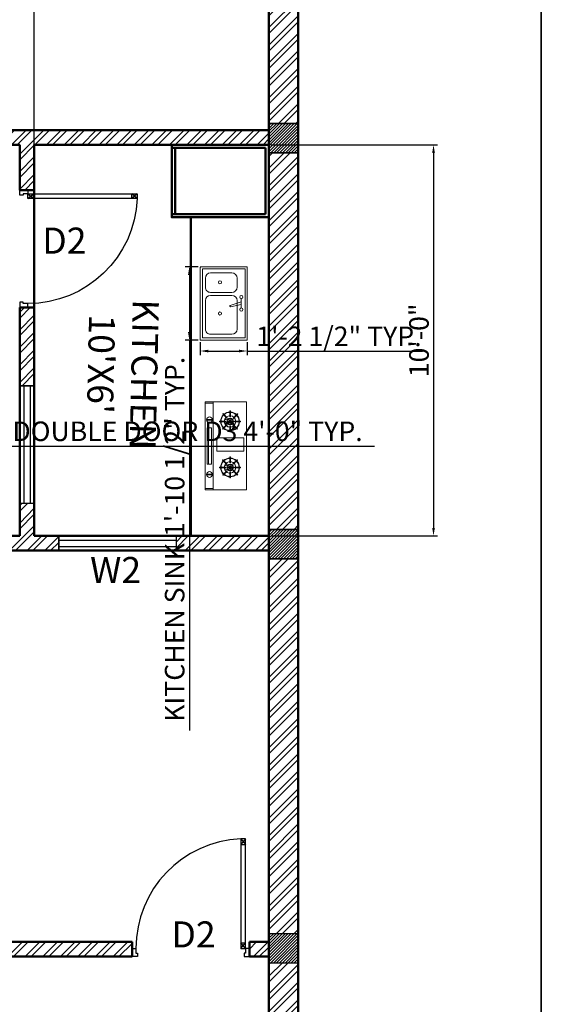
# Model space of a CAD drawing. Units: millimetres. Extents: x 20768 to 23556, y 50760 to 52704.
# Tile 25 of 36: x 21474 to 21634, y 52066 to 52368. Entities that reach past the tile are written whole.
import ezdxf

# ---------------------------------------------------------------- set-up
doc = ezdxf.new("R2010")
doc.units = ezdxf.units.MM
for name, color, linetype, lineweight in [('A-ANNO-TTLB', 7, 'Continuous', 35), ('A-AREA-IDEN', 40, 'Continuous', 18), ('A-DOOR', 3, 'Continuous', 25), ('A-FURN', 8, 'Continuous', 18), ('A-GLAZ', 4, 'Continuous', 25), ('A-WALL', 7, 'Continuous', 50), ('A-WALL-PATT', 8, 'Continuous', 13), ('S-ANNO-DIMS', 2, 'Continuous', 18), ('S-COLS', 20, 'Continuous', 35)]:
    doc.layers.add(name, color=color, linetype=linetype, lineweight=lineweight)
doc.styles.get("Standard").update_dxf_attribs({"font": 'arial.ttf'})
doc.dimstyles.new('ISO-25', dxfattribs={"dimtxt": 6, "dimasz": 2.5, "dimexe": 1.25, "dimexo": 0.625, "dimtad": 1, "dimdec": 0, "dimlunit": 3, "dimtxsty": 'Standard', "dimcen": 2.5, "dimadec": 0, "dimazin": 0, "dimtfac": 1, "dimtdec": 0, "dimtmove": 0, "dimatfit": 3, "dimfxl": 1, "dimarcsym": 0})
pattern_1 = [(45, (-37.4434, 0), (-2.69407684, 2.69407684), []), (45, (-35.6473, 0), (-2.69407684, 2.69407684), [])]
pattern_2 = [(45, (345.4904, 0), (-0.449012806, 0.449012806), [])]

# ---------------------------------------------------------------- blocks, each defined once
blk = doc.blocks.new('Puerta 01')
for p, q in [((-0.7745, -0.0264), (-0.7368, -0.0584)), ((-0.7745, -0.0584), (-0.7368, -0.0264)), ((-0.7368, -0.0584), (-0.7368, -0.0264)), ((-0.028, -0.0584), (-0.0657, -0.0264)), ((-0.028, -0.0264), (-0.0657, -0.0584)), ((-0.0657, -0.0584), (-0.0657, -0.0264))]:
    blk.add_line(p, q)
for points in [[(-0.028, 0), (-0.028, -0.0264), (0.004, -0.0264), (0.004, -0.036), (0.028, -0.036), (0.028, 0)], [(-0.028, -0.0264), (-0.7745, -0.0264), (-0.7745, -0.0584), (-0.028, -0.0584)], [(0.004, -0.7736), (0.004, -0.764), (0.028, -0.764), (0.028, -0.8), (-0.028, -0.8), (-0.028, -0.7736)]]:
    blk.add_lwpolyline(points, close=True)
blk.add_arc((-0.028, -0.0264), 0.7472, 182.45453, 270)
blk = doc.blocks.new('A$C46C9437A')
for p, q in [((0, 416.4), (0, 0.8)), ((884.8, 416.4), (0, 416.4)), ((884.8, 0.8), (884.8, 416.4)), ((163, 281.2), (120.3, 323.9)), ((166.8, 285), (124.1, 327.7)), ((194.5, 296.3), (194.5, 356.7)), ((199.9, 296.2), (199.9, 356.6)), ((228.4, 283.6), (271.1, 326.3)), ((232.1, 279.7), (274.9, 322.4)), ((495.4, 390.2), (361.5, 390.2)), ((361.5, 390.2), (361.5, 118)), ((495.4, 118), (495.4, 390.2)), ((624.8, 279.7), (582.1, 322.4)), ((628.5, 283.6), (585.8, 326.3)), ((657, 296.2), (657, 356.6)), ((662.4, 296.3), (662.4, 356.7)), ((690.1, 285), (732.8, 327.7)), ((693.9, 281.2), (736.6, 323.9)), ((151.4, 249.7), (91, 249.7)), ((151.6, 255.1), (91.1, 255.1)), ((160.6, 223.4), (117.7, 180.6)), ((164.1, 219.3), (121.4, 176.6)), ((171.6, 252.1), (165.7, 252.1)), ((165.7, 252.1), (165.7, 251.1)), ((165.7, 251.1), (171.6, 251.1)), ((171.6, 251.1), (171.6, 252.1)), ((181.4, 195.8), (172.2, 230.6)), ((194.5, 205.4), (194.5, 145)), ((197.3, 281.9), (196.3, 281.9)), ((196.3, 281.9), (196.3, 276.4)), ((196.3, 276.4), (197.3, 276.4)), ((197.3, 226.1), (196.3, 226.1)), ((196.3, 226.1), (196.3, 220.6)), ((196.3, 220.6), (197.3, 220.6)), ((197.3, 276.4), (197.3, 281.9)), ((197.3, 220.6), (197.3, 226.1)), ((199.9, 205.4), (199.9, 145)), ((212, 195.1), (222.8, 232)), ((227.3, 252.1), (221.4, 252.1)), ((221.4, 252.1), (221.4, 251.1)), ((221.4, 251.1), (227.3, 251.1)), ((227.2, 216.9), (269.9, 174.2)), ((227.3, 251.1), (227.3, 252.1)), ((231, 220.8), (273.7, 178.1)), ((242.2, 255.1), (302.6, 255.1)), ((242.4, 249.7), (302.7, 249.7)), ((614.6, 249.7), (554.2, 249.7)), ((614.7, 255.1), (554.3, 255.1)), ((625.9, 220.8), (583.2, 178.1)), ((629.7, 216.9), (587, 174.2)), ((629.6, 251.1), (629.6, 252.1)), ((629.6, 252.1), (635.6, 252.1)), ((635.6, 251.1), (629.6, 251.1)), ((644.9, 195.1), (634.1, 232)), ((635.6, 252.1), (635.6, 251.1)), ((657, 205.4), (657, 145)), ((659.6, 276.4), (659.6, 281.9)), ((659.6, 281.9), (660.7, 281.9)), ((660.7, 276.4), (659.6, 276.4)), ((659.6, 220.6), (659.6, 226.1)), ((659.6, 226.1), (660.7, 226.1)), ((660.7, 220.6), (659.6, 220.6)), ((660.7, 281.9), (660.7, 276.4)), ((660.7, 226.1), (660.7, 220.6)), ((662.4, 205.4), (662.4, 145)), ((675.5, 195.8), (684.7, 230.6)), ((685.3, 251.1), (685.3, 252.1)), ((685.3, 252.1), (691.3, 252.1)), ((691.3, 251.1), (685.3, 251.1)), ((691.3, 252.1), (691.3, 251.1)), ((692.8, 219.3), (735.5, 176.6)), ((696.3, 223.4), (739.2, 180.6)), ((705.3, 255.1), (765.8, 255.1)), ((705.5, 249.7), (765.9, 249.7)), ((361.5, 118), (495.4, 118)), ((0, 82.1), (884.8, 82.1)), ((0, 0.8), (884.8, 0.8)), ((11.9, 0), (11.9, 81.7)), ((184.5, 70.7), (176.8, 70.7)), ((176.8, 70.7), (176.8, 15.6)), ((176.8, 15.6), (184.5, 15.6)), ((184.5, 15.6), (184.5, 70.7)), ((628.6, 65.2), (261.1, 65.2)), ((261.1, 65.2), (261.1, 20.8)), ((628.6, 32.6), (261.1, 32.6)), ((261.1, 20.8), (628.6, 20.8)), ((628.6, 20.8), (628.6, 65.2)), ((735.8, 70.7), (728.1, 70.7)), ((728.1, 70.7), (728.1, 15.6)), ((728.1, 15.6), (735.8, 15.6)), ((735.8, 15.6), (735.8, 70.7)), ((872.3, 0), (872.3, 81.7))]:
    blk.add_line(p, q)
for centre, radius in [((196.7, 251.4), 32.5), ((196.7, 251.4), 30.7), ((173.8, 251.8), 2.11), ((180.2, 236.2), 2.11), ((180.6, 267.5), 2.11), ((196.2, 251.6), 14.5), ((196.2, 251.6), 12.7), ((196, 251.9), 4.75), ((196.7, 274.5), 2.11), ((196.7, 228.2), 2.11), ((211.9, 235.8), 2.11), ((212.3, 267), 2.11), ((218.6, 251.8), 2.11), ((660.3, 251.4), 32.5), ((660.3, 251.4), 30.7), ((638.3, 251.8), 2.11), ((644.6, 267), 2.11), ((645, 235.8), 2.11), ((660.7, 251.6), 14.5), ((660.7, 251.6), 12.7), ((660.9, 251.9), 4.75), ((660.3, 274.5), 2.11), ((660.3, 228.2), 2.11), ((676.3, 267.5), 2.11), ((676.7, 236.2), 2.11), ((683.1, 251.8), 2.11), ((180.1, 43.9), 29), ((731.4, 43.9), 29)]:
    blk.add_circle(centre, radius)
for centre, radius, start, end in [((196.9, 250.8), 94.6, 136.5182, 177.42683), ((196.9, 250.8), 91, 136.57828, 177.32495), ((196.9, 250.8), 105.8, 133.43323, 136.35675), ((196.9, 250.8), 94.6, 91.4483, 133.24678), ((196.9, 250.8), 91, 91.50561, 133.17739), ((196.9, 250.8), 57.2, 92.39717, 175.73928), ((196.5, 239.1), 117.6, 88.37076, 91.29429), ((196.9, 250.8), 94.6, 45.52997, 88.17687), ((196.9, 250.8), 91, 45.55094, 88.10471), ((196.9, 250.8), 57.2, 45.87705, 86.98209), ((196.9, 250.8), 91, 2.67505, 42.14937), ((196.9, 250.8), 94.6, 2.57317, 42.25795), ((196.9, 250.8), 105.8, 42.54967, 45.47362), ((660, 250.8), 94.6, 137.74205, 177.42683), ((660, 250.8), 91, 137.85063, 177.32495), ((660, 250.8), 105.8, 134.52638, 137.45033), ((660, 250.8), 94.6, 91.82313, 134.47003), ((660, 250.8), 91, 91.89529, 134.44906), ((660, 250.8), 57.2, 93.01791, 134.12295), ((660.4, 239.1), 117.6, 88.70571, 91.62924), ((660, 250.8), 94.6, 46.75322, 88.5517), ((660, 250.8), 91, 46.82261, 88.49439), ((660, 250.8), 57.2, 4.26072, 87.60283), ((660, 250.8), 91, 2.67505, 43.42172), ((660, 250.8), 94.6, 2.57317, 43.4818), ((660, 250.8), 105.8, 43.64325, 46.56677), ((208.6, 250.4), 117.6, 177.70057, 180.33206), ((196.9, 250.8), 94.6, 180.69868, 221.19627), ((196.9, 250.8), 91, 180.72632, 221.04554), ((196.9, 250.8), 57.2, 181.15626, 218.6973), ((196.9, 250.8), 45.5, 174.64455, 181.45263), ((196.9, 250.8), 57.2, 224.12295, 267.60283), ((196.9, 250.8), 45.5, 217.07285, 223.89817), ((196.9, 250.8), 45.5, 131.35328, 138.15746), ((196.9, 250.8), 45.5, 86.2077, 93.01198), ((196.9, 250.8), 45.5, 266.98802, 273.7923), ((196.9, 250.8), 57.2, 273.01791, 312.48709), ((196.9, 250.8), 45.5, 311.84254, 318.64672), ((196.9, 250.8), 45.5, 39.2922, 46.10183), ((196.9, 250.8), 57.2, 317.90212, 358.84374), ((196.9, 250.8), 57.2, 4.26072, 40.45928), ((196.9, 250.8), 45.5, 358.54737, 5.35545), ((196.9, 250.8), 91, 316.82261, 359.27368), ((196.9, 250.8), 94.6, 316.75322, 359.30132), ((196.9, 250.8), 105.8, 359.37561, 2.29943), ((660, 250.8), 105.8, 177.70057, 180.62439), ((660, 250.8), 94.6, 180.69868, 223.24678), ((660, 250.8), 91, 180.72632, 223.17739), ((660, 250.8), 57.2, 181.15626, 222.09788), ((660, 250.8), 57.2, 139.54072, 175.73928), ((660, 250.8), 45.5, 174.64455, 181.45263), ((660, 250.8), 57.2, 227.51291, 266.98209), ((660, 250.8), 45.5, 133.89817, 140.7078), ((660, 250.8), 45.5, 221.35328, 228.15746), ((660, 250.8), 45.5, 86.98802, 93.7923), ((660, 250.8), 45.5, 266.2077, 273.01198), ((660, 250.8), 57.2, 272.39717, 315.87705), ((660, 250.8), 45.5, 41.84254, 48.64672), ((660, 250.8), 45.5, 316.10183, 322.92715), ((660, 250.8), 57.2, 321.3027, 358.84374), ((660, 250.8), 45.5, 358.54737, 5.35545), ((660, 250.8), 91, 318.95446, 359.27368), ((660, 250.8), 94.6, 318.80373, 359.30132), ((648.3, 250.4), 117.6, 359.66794, 2.29943), ((196.9, 250.8), 105.8, 221.60119, 224.52638), ((196.9, 250.8), 94.6, 224.47003, 268.5517), ((196.9, 250.8), 91, 224.44906, 268.49439), ((196.9, 250.8), 105.8, 268.70571, 271.62924), ((196.9, 250.8), 91, 271.89529, 313.42172), ((196.9, 250.8), 94.6, 271.82313, 313.4818), ((196.9, 250.8), 105.8, 313.64325, 316.56677), ((660, 250.8), 105.8, 223.43323, 226.35675), ((660, 250.8), 94.6, 226.5182, 268.17687), ((660, 250.8), 91, 226.57828, 268.10471), ((660, 250.8), 105.8, 268.37076, 271.29429), ((660, 250.8), 91, 271.50561, 315.55094), ((660, 250.8), 94.6, 271.4483, 315.52997), ((660, 250.8), 105.8, 315.47362, 318.39881)]:
    blk.add_arc(centre, radius, start, end)
blk = doc.blocks.new('A$C42714C99')
for p, q in [((0, 445), (0, 5)), ((695, 450), (5, 450)), ((20, 430), (20, 20)), ((680, 430), (20, 430)), ((303.8, 392.6), (393.1, 392.6)), ((335.3, 392.6), (369.3, 287.1)), ((360, 392.6), (382, 288.3)), ((680, 20), (680, 430)), ((700, 5), (700, 445)), ((57.3, 98.6), (57.3, 302.2)), ((107.3, 352.2), (194.5, 352.2)), ((244.5, 302.2), (244.5, 98.6)), ((273.1, 98.6), (273.1, 302.2)), ((323.1, 352.2), (594.9, 352.2)), ((644.9, 302.2), (644.9, 98.6)), ((5, 0), (695, 0)), ((20, 20), (680, 20)), ((194.5, 48.6), (107.3, 48.6)), ((594.9, 48.6), (323.1, 48.6))]:
    blk.add_line(p, q)
for centre in [(288.7, 392.6), (408.3, 392.6), (147.5, 188.3), (446.5, 188.3)]:
    blk.add_circle(centre, 15.1)
for centre, radius, start, end in [((5, 445), 5, 90, 180), ((695, 445), 5, 0, 90), ((107.3, 302.2), 50, 90, 180), ((194.5, 302.2), 50, 0, 90), ((323.1, 302.2), 50, 90, 180), ((375.4, 290.3), 6.89, 207.59576, 343.05259), ((594.9, 302.2), 50, 0, 90), ((107.3, 98.6), 50, 180, 270), ((194.5, 98.6), 50, 270, 0), ((323.1, 98.6), 50, 180, 270), ((594.9, 98.6), 50, 270, 0), ((5, 5), 5, 180, 270), ((1, 1), 1, 180, 270), ((695, 5), 5, 270, 0), ((699, 1), 1, 270, 0)]:
    blk.add_arc(centre, radius, start, end)
blk = doc.blocks.new('A$C00DA51E9')
blk.add_blockref('A$C42714C99', (0, 0))
blk = doc.blocks.new('COL-PLAN')
blk.add_line((0, 9), (9, 9))
blk.add_lwpolyline([(9, 9), (0, 9), (0, 0), (9, 0)], close=True)
blk = doc.blocks.new('WIN-PLAN-A')
blk.add_line((36, 4.5), (36, 0))
blk.add_lwpolyline([(36, 4.5), (0, 4.5), (0, 0), (36, 0)], close=True)
blk = doc.blocks.new('*D185')
at = {"layer": 'Defpoints', "color": 0, "transparency": 16777216}
for p in [(21465.84, 52236.99), (21417.84, 52229.79), (21465.84, 52229.79)]:
    blk.add_point(p, dxfattribs=at)
at = {"layer": 'S-ANNO-DIMS', "color": 0, "lineweight": -2, "transparency": 16777216}
for p, q in [((21417.84, 52230.42), (21417.84, 52238.24)), ((21465.84, 52230.42), (21465.84, 52238.24)), ((21420.34, 52236.99), (21463.34, 52236.99)), ((21465.84, 52236.99), (21583.18, 52236.99))]:
    blk.add_line(p, q, dxfattribs=at)
at = {"layer": 'S-ANNO-DIMS', "color": 0, "transparency": 16777216}
for points in [[(21420.34, 52237.41), (21420.34, 52236.58), (21417.84, 52236.99)], [(21463.34, 52237.41), (21463.34, 52236.58), (21465.84, 52236.99)]]:
    blk.add_solid(points, dxfattribs=at)
at = {"layer": 'S-ANNO-DIMS', "color": 0, "transparency": 16777216, "insert": (21525.76, 52240.73), "char_height": 6, "attachment_point": 5}
blk.add_mtext('DOUBLE DOOR D3 4\'-0" TYP.', dxfattribs=at)
blk = doc.blocks.new('*D195')
at = {"layer": 'Defpoints', "color": 0, "transparency": 16777216}
for p in [(21529.68, 52291.94), (21526.32, 52269.49), (21529.68, 52269.49)]:
    blk.add_point(p, dxfattribs=at)
at = {"layer": 'S-ANNO-DIMS', "color": 0, "lineweight": -2, "transparency": 16777216}
for p, q in [((21529.06, 52291.94), (21525.07, 52291.94)), ((21526.32, 52289.44), (21526.32, 52271.99)), ((21529.06, 52269.49), (21525.07, 52269.49)), ((21526.32, 52269.49), (21526.32, 52149.78))]:
    blk.add_line(p, q, dxfattribs=at)
at = {"layer": 'S-ANNO-DIMS', "color": 0, "transparency": 16777216}
for points in [[(21525.9, 52289.44), (21526.73, 52289.44), (21526.32, 52291.94)], [(21525.9, 52271.99), (21526.73, 52271.99), (21526.32, 52269.49)]]:
    blk.add_solid(points, dxfattribs=at)
at = {"layer": 'S-ANNO-DIMS', "color": 0, "transparency": 16777216, "insert": (21522.59, 52208.39), "char_height": 6, "attachment_point": 5, "rotation": 90}
blk.add_mtext('KITCHEN SINK 1\'-10 1/2" TYP.', dxfattribs=at)
blk = doc.blocks.new('*D196')
at = {"layer": 'Defpoints', "color": 0, "transparency": 16777216}
for p in [(21529.68, 52269.49), (21544.11, 52269.49), (21544.11, 52266.13)]:
    blk.add_point(p, dxfattribs=at)
at = {"layer": 'S-ANNO-DIMS', "color": 0, "lineweight": -2, "transparency": 16777216}
for p, q in [((21529.68, 52268.87), (21529.68, 52264.88)), ((21544.11, 52268.87), (21544.11, 52264.88)), ((21532.18, 52266.13), (21541.61, 52266.13)), ((21544.11, 52266.13), (21597.85, 52266.13))]:
    blk.add_line(p, q, dxfattribs=at)
at = {"layer": 'S-ANNO-DIMS', "color": 0, "transparency": 16777216}
for points in [[(21532.18, 52266.54), (21532.18, 52265.71), (21529.68, 52266.13)], [(21541.61, 52266.54), (21541.61, 52265.71), (21544.11, 52266.13)]]:
    blk.add_solid(points, dxfattribs=at)
at = {"layer": 'S-ANNO-DIMS', "color": 0, "transparency": 16777216, "insert": (21572.23, 52269.85), "char_height": 6, "attachment_point": 5}
blk.add_mtext('1\'-2 1/2" TYP.', dxfattribs=at)
blk = doc.blocks.new('*D214')
at = {"layer": 'Defpoints', "color": 0, "transparency": 16777216}
for p in [(21550.74, 52329.4), (21550.74, 52209.4), (21601.27, 52209.4)]:
    blk.add_point(p, dxfattribs=at)
at = {"layer": 'S-ANNO-DIMS', "color": 0, "lineweight": -2, "transparency": 16777216}
for p, q in [((21551.37, 52329.4), (21602.52, 52329.4)), ((21601.27, 52326.9), (21601.27, 52211.9)), ((21551.37, 52209.4), (21602.52, 52209.4))]:
    blk.add_line(p, q, dxfattribs=at)
at = {"layer": 'S-ANNO-DIMS', "color": 0, "transparency": 16777216}
for points in [[(21600.86, 52326.9), (21601.69, 52326.9), (21601.27, 52329.4)], [(21600.86, 52211.9), (21601.69, 52211.9), (21601.27, 52209.4)]]:
    blk.add_solid(points, dxfattribs=at)
at = {"layer": 'S-ANNO-DIMS', "color": 0, "transparency": 16777216, "insert": (21597.58, 52269.4), "char_height": 6, "attachment_point": 5, "rotation": 90}
blk.add_mtext('10\'-0"', dxfattribs=at)
blk = doc.blocks.new('*D216')
at = {"layer": 'Defpoints', "color": 0, "transparency": 16777216}
for p in [(21550.74, 52564.4), (21478.74, 52209.4), (21550.74, 52209.4)]:
    blk.add_point(p, dxfattribs=at)
at = {"layer": 'S-ANNO-DIMS', "color": 0, "lineweight": -2, "transparency": 16777216}
for p, q in [((21478.74, 52210.02), (21478.74, 52565.65)), ((21481.24, 52564.4), (21548.24, 52564.4)), ((21550.74, 52210.02), (21550.74, 52565.65))]:
    blk.add_line(p, q, dxfattribs=at)
at = {"layer": 'S-ANNO-DIMS', "color": 0, "transparency": 16777216}
for points in [[(21481.24, 52564.81), (21481.24, 52563.98), (21478.74, 52564.4)], [(21548.24, 52564.81), (21548.24, 52563.98), (21550.74, 52564.4)]]:
    blk.add_solid(points, dxfattribs=at)
at = {"layer": 'S-ANNO-DIMS', "color": 0, "transparency": 16777216, "insert": (21514.74, 52568.09), "char_height": 6, "attachment_point": 5}
blk.add_mtext('6\'-0"', dxfattribs=at)

msp = doc.modelspace()

# ---------------------------------------------------------------- hatches: boundary and pattern name
at = {"layer": 'A-WALL-PATT'}
h = msp.add_hatch(dxfattribs=at)
h.set_pattern_fill('ANSI32', color=256, scale=0.4)
h.set_pattern_definition(pattern_1)
h.paths.add_polyline_path([(21559.74, 52513.9), (21550.74, 52513.9), (21550.74, 52335.9), (21559.74, 52335.9)])
h = msp.add_hatch(dxfattribs=at)
h.set_pattern_fill('ANSI31', color=256, scale=0.2)
h.set_pattern_definition(pattern_2)
h.paths.add_polyline_path([(21559.74, 52335.9), (21550.74, 52335.9), (21550.74, 52326.9), (21559.74, 52326.9)])
h = msp.add_hatch(dxfattribs=at)
h.set_pattern_fill('ANSI32', color=256, scale=0.4)
h.set_pattern_definition(pattern_1)
h.paths.add_polyline_path([(21550.74, 52333.9), (21444.64, 52333.9), (21444.64, 52329.4), (21474.24, 52329.4), (21474.24, 52315.5), (21476.76, 52315.5), (21478.74, 52315.5), (21478.74, 52329.4), (21550.74, 52329.4)])
h = msp.add_hatch(dxfattribs=at)
h.set_pattern_fill('ANSI32', color=256, scale=0.4)
h.set_pattern_definition(pattern_1)
h.paths.add_polyline_path([(21559.74, 52326.9), (21550.74, 52326.9), (21550.74, 52307.13), (21550.74, 52211.4), (21559.74, 52211.4)])
h = msp.add_hatch(dxfattribs=at)
h.set_pattern_fill('ANSI32', color=256, scale=0.4)
h.set_pattern_definition(pattern_1)
h.paths.add_polyline_path([(21478.74, 52279.5), (21474.24, 52279.5), (21474.24, 52255.5), (21478.74, 52255.5)])
h = msp.add_hatch(dxfattribs=at)
h.set_pattern_fill('ANSI32', color=256, scale=0.4)
h.set_pattern_definition(pattern_1)
h.paths.add_polyline_path([(21486.24, 52209.4), (21478.74, 52209.4), (21478.74, 52219.5), (21474.24, 52219.5), (21474.24, 52209.4), (21465.84, 52209.4), (21465.84, 52204.9), (21486.24, 52204.9)])
h = msp.add_hatch(dxfattribs=at)
h.set_pattern_fill('ANSI31', color=256, scale=0.2)
h.set_pattern_definition(pattern_2)
h.paths.add_polyline_path([(21559.74, 52211.4), (21550.74, 52211.4), (21550.74, 52202.4), (21559.74, 52202.4)])
h = msp.add_hatch(dxfattribs=at)
h.set_pattern_fill('ANSI32', color=256, scale=0.4)
h.set_pattern_definition(pattern_1)
h.paths.add_polyline_path([(21550.74, 52209.4), (21522.24, 52209.4), (21522.24, 52204.9), (21550.74, 52204.9)])
h = msp.add_hatch(dxfattribs=at)
h.set_pattern_fill('ANSI32', color=256, scale=0.4)
h.set_pattern_definition(pattern_1)
h.paths.add_polyline_path([(21559.74, 52202.4), (21550.74, 52202.4), (21550.74, 52087.4), (21559.74, 52087.4)])
h = msp.add_hatch(dxfattribs=at)
h.set_pattern_fill('ANSI32', color=256, scale=0.4)
h.set_pattern_definition(pattern_1)
h.paths.add_polyline_path([(21508.74, 52084.9), (21411.24, 52084.9), (21411.24, 52090.9), (21406.74, 52090.9), (21406.74, 52084.9), (21334.74, 52084.9), (21334.74, 52080.4), (21508.74, 52080.4)])
h = msp.add_hatch(dxfattribs=at)
h.set_pattern_fill('ANSI31', color=256, scale=0.2)
h.set_pattern_definition([(45, (-37.4434, 0), (-0.449012806, 0.449012806), [])])
h.paths.add_polyline_path([(21559.74, 52087.4), (21550.74, 52087.4), (21550.74, 52078.62), (21559.74, 52078.62)])
h = msp.add_hatch(dxfattribs=at)
h.set_pattern_fill('ANSI32', color=256, scale=0.4)
h.set_pattern_definition(pattern_1)
h.paths.add_polyline_path([(21550.74, 52084.9), (21544.74, 52084.9), (21544.74, 52080.4), (21550.74, 52080.4)])
h = msp.add_hatch(dxfattribs=at)
h.set_pattern_fill('ANSI32', color=256, scale=0.4)
h.set_pattern_definition(pattern_1)
h.paths.add_polyline_path([(21559.74, 52078.62), (21550.74, 52078.62), (21550.74, 51902.4), (21559.74, 51902.4)])

# ---------------------------------------------------------------- linework, layer by layer
at = {"layer": 'A-ANNO-TTLB'}
msp.add_line((21634.36, 52703.98), (21634.36, 51623.53), dxfattribs=at)
at = {"layer": 'A-GLAZ'}
for p, q in [((21475.49, 52255.5), (21475.49, 52219.5)), ((21477.49, 52255.5), (21477.49, 52219.5)), ((21474.24, 52219.5), (21478.74, 52219.5)), ((21486.24, 52208.15), (21522.24, 52208.15)), ((21522.24, 52209.4), (21522.24, 52204.9)), ((21486.24, 52206.15), (21522.24, 52206.15))]:
    msp.add_line(p, q, dxfattribs=at)
at = {"layer": 'A-WALL'}
for p, q in [((21559.74, 52522.9), (21559.74, 51829.9)), ((21550.74, 52513.9), (21550.74, 51834.4)), ((21384.64, 52333.9), (21550.74, 52333.9)), ((21384.64, 52329.4), (21474.24, 52329.4)), ((21474.24, 52329.4), (21474.24, 52315.5)), ((21478.74, 52329.4), (21478.74, 52315.5)), ((21478.74, 52329.4), (21550.74, 52329.4)), ((21549.74, 52328.4), (21520.93, 52328.4)), ((21521.93, 52328.4), (21521.93, 52308.13)), ((21549.74, 52308.13), (21549.74, 52328.4)), ((21474.24, 52315.5), (21478.74, 52315.5)), ((21478.74, 52315.5), (21478.74, 52279.5)), ((21520.93, 52308.13), (21549.74, 52308.13)), ((21526.74, 52307.13), (21526.74, 52209.4)), ((21526.74, 52307.13), (21550.74, 52307.13)), ((21474.24, 52279.5), (21474.24, 52209.4)), ((21474.24, 52279.5), (21478.74, 52279.5)), ((21478.74, 52279.5), (21478.74, 52209.4)), ((21465.24, 52209.4), (21474.24, 52209.4)), ((21478.74, 52209.4), (21550.74, 52209.4)), ((21465.84, 52204.9), (21550.74, 52204.9)), ((21411.24, 52084.9), (21508.74, 52084.9)), ((21508.74, 52084.9), (21508.74, 52080.4)), ((21544.74, 52084.9), (21544.74, 52080.4)), ((21544.74, 52084.9), (21550.74, 52084.9)), ((21334.74, 52080.4), (21508.74, 52080.4)), ((21544.74, 52080.4), (21550.74, 52080.4))]:
    msp.add_line(p, q, dxfattribs=at)
msp.add_lwpolyline([(21550.74, 52329.4), (21520.93, 52329.4), (21520.93, 52307.13), (21550.74, 52307.13)], close=True, dxfattribs=at)
at = {"layer": 'S-COLS'}
msp.add_line((21550.74, 52326.9), (21559.74, 52326.9), dxfattribs=at)

# ---------------------------------------------------------------- block references
at = {"layer": 'A-DOOR', "extrusion": (0, 0, -1), "xscale": 45.00000000000063, "yscale": 45.00000000000063, "zscale": -45.00000000000063}
msp.add_blockref('Puerta 01', (-21475.5, 52315.5), dxfattribs=at)
at = {"layer": 'A-DOOR', "xscale": 45.00000000000063, "yscale": 45.00000000000063, "zscale": 45.00000000000063, "rotation": 270.0000000116385}
msp.add_blockref('Puerta 01', (21544.74, 52081.66), dxfattribs=at)
at = {"layer": 'A-FURN', "rotation": 270}
for name, p, xscale, yscale, zscale in [('A$C00DA51E9', (21529.68, 52291.94), 0.032067883861812, 0.032067883861812, 0.032067883861812), ('A$C46C9437A', (21531.17, 52250.54), 0.0304817367471025, 0.0304817367471025, 0.0304817367471025)]:
    msp.add_blockref(name, p, dxfattribs=dict(at, xscale=xscale, yscale=yscale, zscale=zscale))
at = {"layer": 'A-GLAZ', "rotation": 89.99999999995023}
msp.add_blockref('WIN-PLAN-A', (21478.74, 52219.5), dxfattribs=at)
at = {"layer": 'A-GLAZ', "extrusion": (0, 0, -1), "zscale": -1}
msp.add_blockref('WIN-PLAN-A', (-21522.24, 52204.9), dxfattribs=at)
at = {"layer": 'S-COLS'}
for p in [(21550.74, 52326.9), (21550.74, 52202.4)]:
    msp.add_blockref('COL-PLAN', p, dxfattribs=at)
at = {"layer": 'S-COLS', "rotation": 359.2862440568853}
msp.add_blockref('COL-PLAN', (21550.66, 52078.53), dxfattribs=at)

# ---------------------------------------------------------------- texts
at = {"layer": 'A-AREA-IDEN', "char_height": 8, "attachment_point": 1}
for s, insert in [(' D2', (21478.74, 52303.98)), ('W2', (21495.86, 52202.97)), (' D2', (21518.38, 52091.2))]:
    msp.add_mtext_dynamic_manual_height_columns(s, width=27.5349, gutter_width=12.5, heights=[0], dxfattribs=dict(at, insert=insert))
at = {"layer": 'A-AREA-IDEN', "insert": (21516.99, 52281.86), "char_height": 8, "attachment_point": 1, "rotation": 268.7537}
msp.add_mtext_dynamic_manual_height_columns("KITCHEN\\P  10'X6'", width=49.9521, gutter_width=12.5, heights=[0], dxfattribs=at)

# ---------------------------------------------------------------- dimensions: what is measured, and where the dimension line sits
at = {"layer": 'S-ANNO-DIMS'}
dim = msp.add_linear_dim(base=(21550.74, 52564.4), p1=(21478.74, 52209.4), p2=(21550.74, 52209.4), dimstyle='ISO-25', override={"dimdec": 1, "dimlfac": 1, "dimrnd": 0, "dimzin": 1, "dimdsep": 46, "dimlunit": 4, "dimfrac": 2}, dxfattribs=at)
dim.commit()
dim.dimension.update_dxf_attribs({"geometry": '*D216', "text_midpoint": (21514.74, 52568.09)})
dim = msp.add_linear_dim(base=(21601.27, 52209.4), p1=(21550.74, 52329.4), p2=(21550.74, 52209.4), angle=90, dimstyle='ISO-25', override={"dimdec": 1, "dimlfac": 1, "dimrnd": 0, "dimzin": 1, "dimdsep": 46, "dimlunit": 4, "dimfrac": 2}, dxfattribs=at)
dim.commit()
dim.dimension.update_dxf_attribs({"geometry": '*D214', "text_midpoint": (21597.58, 52269.4)})
dim = msp.add_linear_dim(base=(21526.3152, 52269.4939), p1=(21529.6824, 52291.9414), p2=(21529.6824, 52269.4939), angle=270, text='KITCHEN SINK <> TYP.', dimstyle='ISO-25', override={"dimdec": 1, "dimrnd": 0, "dimzin": 1, "dimlunit": 4, "dimfrac": 2}, dxfattribs=at)
dim.commit()
dim.dimension.update_dxf_attribs({"geometry": '*D195', "text_midpoint": (21522.5879, 52208.3887)})
for base, p1, p2, text, picture, middle in [((21544.11, 52266.13), (21529.68, 52269.49), (21544.11, 52269.49), '<> TYP.', '*D196', (21572.23, 52269.85)), ((21465.84, 52236.99), (21417.84, 52229.79), (21465.84, 52229.79), 'DOUBLE DOOR D3 <> TYP.', '*D185', (21525.76, 52240.73))]:
    dim = msp.add_linear_dim(base=base, p1=p1, p2=p2, text=text, dimstyle='ISO-25', override={"dimdec": 1, "dimrnd": 0, "dimzin": 1, "dimlunit": 4, "dimfrac": 2}, dxfattribs=at)
    dim.commit()
    dim.dimension.update_dxf_attribs({"geometry": picture, "text_midpoint": middle})

doc.saveas('drawing.dxf')
